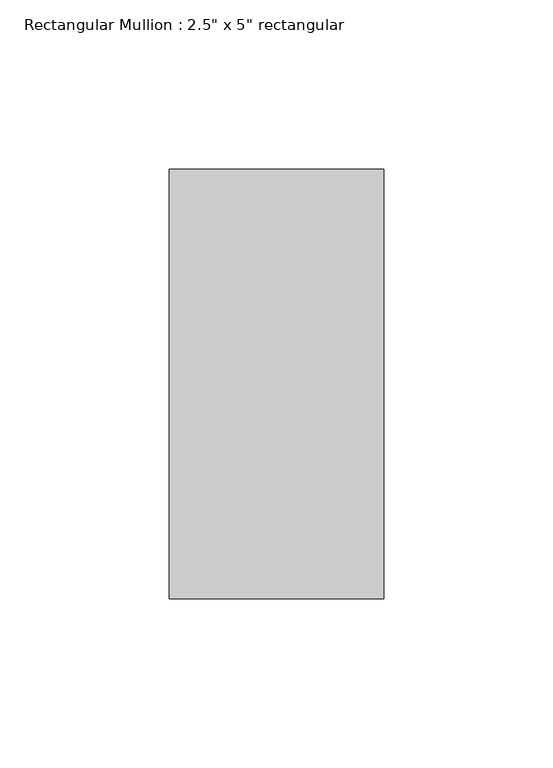
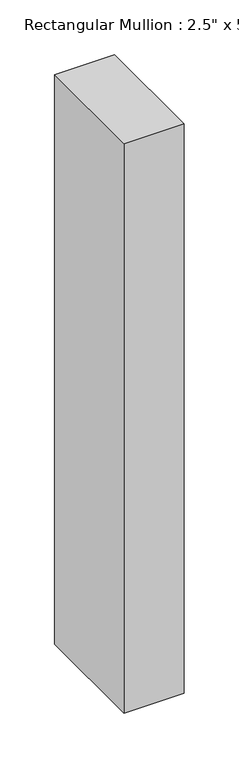
"""IFC4 building model written with IfcOpenShell, lengths in millimetres: member geometry."""

from ifc_helpers import new_model, si_unit, frame, origin, place, context, project, spatial, polyline, outline, extrude, source, transform, mapped, element, save


def member_5e365d0c(model_context):
    return source(origin(), model_context, "Body", "SweptSolid", [
        extrude(outline(polyline([(0.0, 63.5), (0.0, -63.5), (-63.5, -63.5), (-63.5, 63.5), (0.0, 63.5)])), frame((0.0, 0.0, -635.0), z_axis=(0.0, 0.0, 1.0), x_axis=(1.0, 0.0, 0.0)), (0.0, 0.0, 1.0), 635.0),
    ])


if __name__ == "__main__":
    model = new_model("IFC4")
    model_context = context("Model", 3, world=origin())
    ifc_project = project(units=[si_unit("LENGTHUNIT", "METRE", prefix="MILLI")], contexts=[model_context])
    site = spatial("IfcSite", under=ifc_project)
    building = spatial("IfcBuilding", under=site)
    placement = place(None, origin())
    member_shape = member_5e365d0c(model_context)
    element("IfcMember", 1, ObjectType="Rectangular Mullion : 2.5\" x 5\" rectangular", at=placement, inside=building, context=model_context, shape_type="MappedRepresentation", body=[
        mapped(member_shape, transform((0.0, 0.0, 0.0), x_axis=(1.0, 0.0, 0.0), y_axis=(0.0, 1.0, 0.0), z_axis=(0.0, 0.0, 1.0))),
    ])
    save(model, "model.ifc")

# Revit data of these elements
# Type "Rectangular Mullion : 2.5\" x 5\" rectangular"
#   built-in parameter 1007304 = 0.416667 (stored number, unit not read)
#   built-in parameter 1007301 = 0.104167 (stored number, unit not read)
#   built-in parameter 1007300 = 0.104167 (stored number, unit not read)
# Element 1 (IfcMember, "Rectangular Mullion : 2.5\" x 5\" rectangular")
#   Materials on its faces: "Iron, Ductile"
# Materials
#   "Iron, Ductile": class "Metal", colour RGB 0 0 0, transparency 0, Description = "Ductile cast iron", Cost = 0
